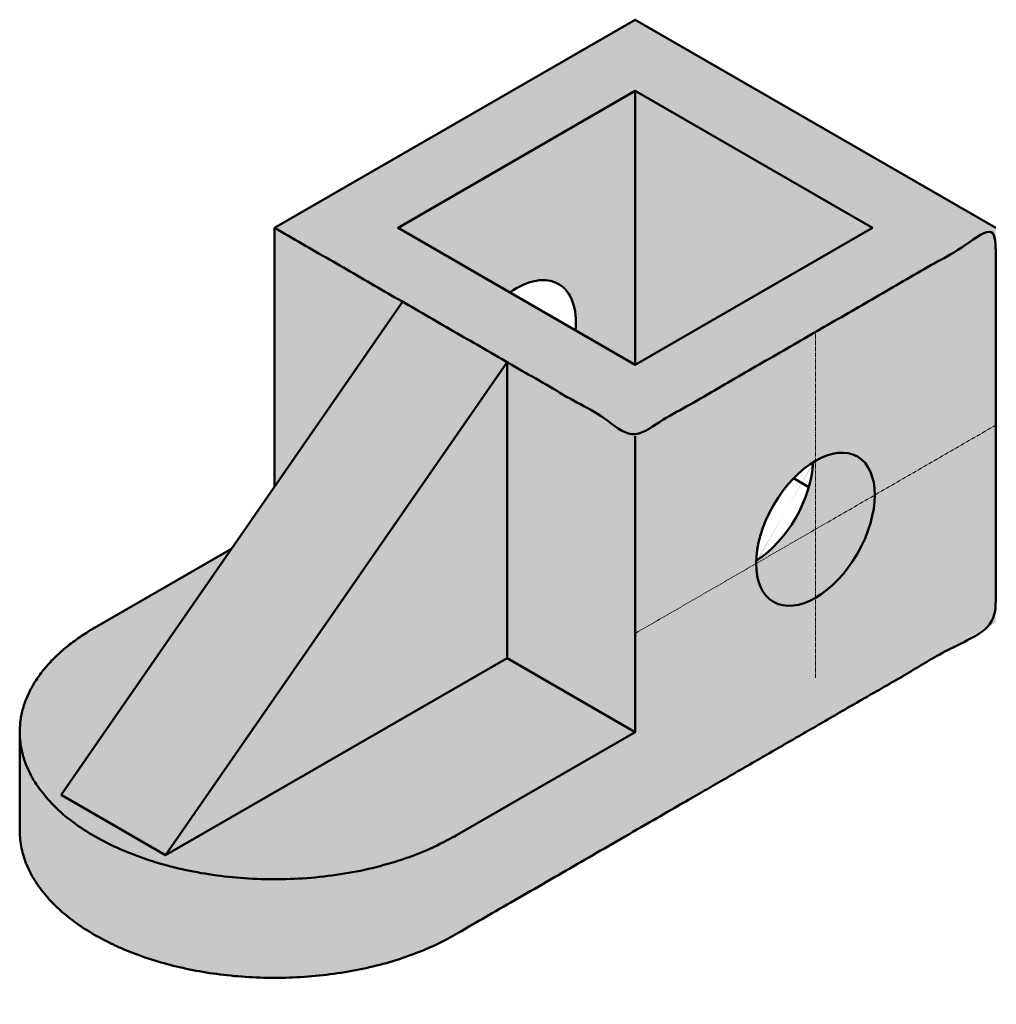
# Model space of a CAD drawing. Units: millimetres. Extents: x -10 to 168, y 10 to 190.
import ezdxf

# ---------------------------------------------------------------- set-up
doc = ezdxf.new("R2010")
doc.units = ezdxf.units.MM
doc.header["$MEASUREMENT"] = 0
doc.linetypes.add('CENTER2', pattern=[1.125, 0.75, -0.125, 0.125, -0.125])
for name, color, linetype, lineweight in [('M-CNTR', 4, 'CENTER2', 18), ('M-HATC', 7, 'Continuous', 18), ('M-OUTL', 7, 'Continuous', 50)]:
    doc.layers.add(name, color=color, linetype=linetype, lineweight=lineweight)

msp = doc.modelspace()

# ---------------------------------------------------------------- hatches: boundary and pattern name
at = {"layer": 'M-HATC'}
h = msp.add_hatch(color=256, dxfattribs=at)
h.set_gradient(color1=(229, 232, 120), color2=(229, 232, 120), tint=1)
edge = h.paths.add_edge_path()
edge.add_line((102.0273422709656, 189.9473373900985), (36.2094115833483, 151.9473373900985))
edge.add_spline(control_points=[(36.20941158334833, 151.9473373900985), (47.88458083858976, 145.2066752777504), (59.55975009383122, 138.4660131654023)], knot_values=[7.001422800068761, 7.001422800068761, 7.001422800068761, 7.356194490192344, 7.356194490192344, 7.356194490192344], weights=[1, 1, 1], degree=2, periodic=0)
edge.add_spline(control_points=[(59.55975009383122, 138.4660131654023), (64.33906351049411, 135.7066752777504), (69.11837692715702, 132.9473373900985)], knot_values=[6.856194490192344, 6.856194490192344, 6.856194490192344, 7.001422800068761, 7.001422800068761, 7.001422800068761], weights=[1, 1, 1], degree=2, periodic=0)
edge.add_spline(control_points=[(69.11837692715702, 132.9473373900985), (73.88151664797141, 130.1973373900985), (78.6446563687858, 127.4473373900985)], knot_values=[6.711457648087082, 6.711457648087082, 6.711457648087082, 6.856194490192344, 6.856194490192344, 6.856194490192344], weights=[1, 1, 1], degree=2, periodic=0)
edge.add_spline(control_points=[(78.6446563687858, 127.4473373900985), (90.33599931987573, 120.6973373900985), (102.0273422709657, 113.9473373900985)], knot_values=[6.356194490192344, 6.356194490192344, 6.356194490192344, 6.711457648087082, 6.711457648087082, 6.711457648087082], weights=[1, 1, 1], degree=2, periodic=0)
edge.add_spline(control_points=[(102.0273422709657, 113.9473373900985), (118.48182494287, 123.4473373900985), (134.9363076147743, 132.9473373900985)], knot_values=[5.856194490192345, 5.856194490192345, 5.856194490192345, 6.356194490192345, 6.356194490192345, 6.356194490192345], weights=[1, 1, 1], degree=2, periodic=0)
edge.add_spline(control_points=[(134.9363076147743, 132.9473373900985), (151.3907902866787, 142.4473373900985), (167.845272958583, 151.9473373900985)], knot_values=[5.356194490192345, 5.356194490192345, 5.356194490192345, 5.856194490192345, 5.856194490192345, 5.856194490192345], weights=[1, 1, 1], degree=2, periodic=0)
edge.add_line((167.845272958583, 151.9473373900985), (102.0273422709656, 189.9473373900985))
h.paths.add_polyline_path([(145.3286124601876, 151.9473373900985), (102.0273422709657, 126.9473373900985), (58.72607208174374, 151.9473373900985), (102.0273422709656, 176.9473373900985)], flags=16)
edge = h.paths.add_edge_path()
edge.add_spline(control_points=[(167.845272958583, 115.9473373900985), (167.845272958583, 133.9473373900985), (167.845272958583, 151.9473373900985)], knot_values=[4.856194490192345, 4.856194490192345, 4.856194490192345, 5.356194490192345, 5.356194490192345, 5.356194490192345], weights=[1, 1, 1], degree=2, periodic=0)
edge.add_spline(control_points=[(167.845272958583, 151.9473373900985), (151.3907902866787, 142.4473373900985), (134.9363076147743, 132.9473373900985)], knot_values=[5.356194490192345, 5.356194490192345, 5.356194490192345, 5.856194490192345, 5.856194490192345, 5.856194490192345], weights=[1, 1, 1], degree=2, periodic=0)
edge.add_line((134.9363076147743, 132.9473373900985), (134.9363076147743, 109.4473373900985))
edge.add_ellipse((134.9363076147743, 96.94733739009851), major_axis=(-7.654655446197424, -13.25825214724778), ratio=0.577350269189626, start_angle=149.9999999999999, end_angle=210, ccw=False)
edge.add_line((145.7616251620798, 103.1973373900985), (167.845272958583, 115.9473373900985))
edge = h.paths.add_edge_path()
edge.add_spline(control_points=[(134.9363076147743, 132.9473373900985), (118.48182494287, 123.4473373900985), (102.0273422709657, 113.9473373900985)], knot_values=[5.856194490192345, 5.856194490192345, 5.856194490192345, 6.356194490192345, 6.356194490192345, 6.356194490192345], weights=[1, 1, 1], degree=2, periodic=0)
edge.add_line((102.0273422709656, 113.9473373900985), (102.0273422709657, 77.94733739009851))
edge.add_line((102.0273422709657, 77.94733739009851), (124.1064732416631, 90.6947295995037))
edge.add_ellipse((134.9363076147743, 96.94733739009851), major_axis=(-7.654655446197424, -13.25825214724778), ratio=0.577350269189626, start_angle=327.93073727587256, end_angle=329.99999999999994, ccw=False)
edge.add_ellipse((134.9363076147743, 96.94733739009851), major_axis=(-7.654655446197424, -13.25825214724778), ratio=0.577350269189626, start_angle=212.0692627241274, end_angle=327.93073727587256, ccw=False)
edge.add_line((134.9363076147743, 109.5003097916459), (134.9363076147743, 132.9473373900985))
edge = h.paths.add_edge_path()
edge.add_ellipse((134.9363076147743, 96.94733739009851), major_axis=(-7.654655446197424, -13.25825214724778), ratio=0.577350269189626, start_angle=329.99999999999994, end_angle=389.99999999999994, ccw=False)
edge.add_line((124.1109900674688, 90.69733739009851), (102.0273422709657, 77.94733739009851))
edge.add_line((102.0273422709657, 77.94733739009851), (102.0273422709656, 59.94733739009851))
edge.add_line((102.0273422709656, 59.94733739009851), (69.11837692715771, 40.94733739009922))
edge.add_spline(control_points=[(69.11837692715702, 40.94733739009853), (50.11837692715701, 29.97768227549562), (24.16389425525267, 33.99285471819417), (-1.790588416651686, 38.00802716089272), (-8.745071088556024, 52.99285471819417), (-10.330893529532, 56.409827185539), (-10.33089352953207, 59.9473373900982)], knot_values=[1.78086055689268, 1.78086055689268, 1.78086055689268, 2.828058108089279, 2.828058108089279, 3.875255659285876, 3.875255659285876, 4.141592653589794, 4.141592653589794, 4.141592653589794], weights=[1, 0.8660254037844385, 1, 0.8660254037844385, 1, 0.9659258262890698, 0.9491840326991372], degree=2, periodic=0)
edge.add_spline(control_points=[(-10.33089352953207, 59.94733739009851), (-10.33089352953207, 50.94733739009851), (-10.33089352953207, 41.9473373900985)], knot_values=[0, 0, 0, 1, 1, 1], weights=[1, 1, 1], degree=2, periodic=0)
edge.add_spline(control_points=[(-10.33089352953207, 41.9473373900985), (-10.33089352953208, 23.99333884526288), (18.39920787943271, 17.12264105744734), (47.12930928839751, 10.25194326963181), (69.11837692715702, 22.94733739009852)], knot_values=[1, 1, 1, 2.178097245096171, 2.178097245096171, 3.356194490192345, 3.356194490192345, 3.356194490192345], weights=[1, 0.831469612302545, 1, 0.831469612302545, 1], degree=2, periodic=0)
edge.add_spline(control_points=[(69.11837692715702, 22.94733739009852), (118.48182494287, 51.44733739009851), (167.845272958583, 79.94733739009851)], knot_values=[3.356194490192345, 3.356194490192345, 3.356194490192345, 4.356194490192345, 4.356194490192345, 4.356194490192345], weights=[1, 1, 1], degree=2, periodic=0)
edge.add_spline(control_points=[(167.845272958583, 79.94733739009851), (167.845272958583, 97.94733739009851), (167.845272958583, 115.9473373900985)], knot_values=[4.356194490192345, 4.356194490192345, 4.356194490192345, 4.856194490192345, 4.856194490192345, 4.856194490192345], weights=[1, 1, 1], degree=2, periodic=0)
edge.add_line((167.845272958583, 115.9473373900985), (145.7616251620798, 103.1973373900985))
edge.add_ellipse((134.9363076147743, 96.94733739009851), major_axis=(-7.654655446197424, -13.25825214724778), ratio=0.577350269189626, start_angle=29.999999999999886, end_angle=149.9999999999999, ccw=False)
edge = h.paths.add_edge_path()
edge.add_line((102.0273422709657, 77.94733739009851), (102.0273422709656, 113.9473373900985))
edge.add_spline(control_points=[(102.0273422709657, 113.9473373900985), (90.33599931987573, 120.6973373900985), (78.6446563687858, 127.4473373900985)], knot_values=[6.356194490192345, 6.356194490192345, 6.356194490192345, 6.711457648087082, 6.711457648087082, 6.711457648087082], weights=[1, 1, 1], degree=2, periodic=0)
edge.add_line((78.6446563687858, 127.4473373900985), (78.6446563687858, 73.4473373900985))
edge.add_line((78.6446563687858, 73.4473373900985), (102.0273422709656, 59.94733739009851))
edge.add_line((102.0273422709656, 59.94733739009851), (102.0273422709657, 77.94733739009851))
edge = h.paths.add_edge_path(flags=17)
edge.add_line((78.6446563687858, 73.44733739009848), (16.29082729630624, 37.44733739009851))
edge.add_line((16.29082729630624, 37.44733739009851), (-2.794078978648371, 48.46601316540233))
edge.add_line((-2.794078978648371, 48.46601316540233), (28.33970570199551, 93.4037605810563))
edge.add_line((28.33970570199551, 93.4037605810563), (3.300446239539809, 78.94733739009858))
edge.add_spline(control_points=[(3.300446239539661, 78.94733739009851), (-10.33089352953229, 71.07727970500959), (-10.33089352953207, 59.9473373900982)], knot_values=[1, 1, 1, 1.78086055689268, 1.78086055689268, 1.78086055689268], weights=[1, 0.9000995774953688, 0.9491840326991372], degree=2, periodic=0)
edge.add_spline(control_points=[(-10.33089352953207, 59.9473373900982), (-10.330893529532, 56.409827185539), (-8.745071088556024, 52.99285471819417), (-1.790588416651686, 38.00802716089272), (24.16389425525267, 33.99285471819417), (50.11837692715701, 29.97768227549562), (69.11837692715702, 40.94733739009853)], knot_values=[1.78086055689268, 1.78086055689268, 1.78086055689268, 2.047197551196598, 2.047197551196598, 3.094395102393195, 3.094395102393195, 4.141592653589794, 4.141592653589794, 4.141592653589794], weights=[0.9491840326991372, 0.9659258262890698, 1, 0.8660254037844385, 1, 0.8660254037844385, 1], degree=2, periodic=0)
edge.add_line((69.1183769271493, 40.94733739009451), (102.0273422709656, 59.94733739009851))
edge.add_line((102.0273422709656, 59.94733739009851), (78.6446563687858, 73.44733739009848))
h.paths.add_polyline_path([(78.6446563687858, 73.4473373900985), (78.6446563687858, 127.4473373900985), (16.29082729630627, 37.44733739009851)], flags=17)
edge = h.paths.add_edge_path()
edge.add_spline(control_points=[(78.6446563687858, 127.4473373900985), (73.88151664797141, 130.1973373900985), (69.11837692715702, 132.9473373900985)], knot_values=[6.711457648087082, 6.711457648087082, 6.711457648087082, 6.856194490192345, 6.856194490192345, 6.856194490192345], weights=[1, 1, 1], degree=2, periodic=0)
edge.add_spline(control_points=[(69.11837692715702, 132.9473373900985), (64.33906351049411, 135.7066752777504), (59.55975009383122, 138.4660131654023)], knot_values=[6.856194490192345, 6.856194490192345, 6.856194490192345, 7.001422800068762, 7.001422800068762, 7.001422800068762], weights=[1, 1, 1], degree=2, periodic=0)
edge.add_line((59.55975009383124, 138.4660131654023), (-2.794078978648343, 48.46601316540231))
edge.add_line((-2.794078978648343, 48.46601316540231), (16.29082729630624, 37.44733739009848))
edge.add_line((16.29082729630624, 37.44733739009848), (78.6446563687858, 127.4473373900985))
edge = h.paths.add_edge_path()
edge.add_spline(control_points=[(59.55975009383121, 138.4660131654023), (47.88458083858976, 145.2066752777503), (36.20941158334833, 151.9473373900985)], knot_values=[7.001422800068762, 7.001422800068762, 7.001422800068762, 7.356194490192345, 7.356194490192345, 7.356194490192345], weights=[1, 1, 1], degree=2, periodic=0)
edge.add_line((36.20941158334833, 151.9473373900985), (36.2094115833483, 104.7627026036618))
edge.add_line((36.2094115833483, 104.7627026036618), (59.55975009383121, 138.4660131654023))
edge = h.paths.add_edge_path(flags=16)
edge.add_line((102.0273422709656, 176.9473373900985), (58.72607208174371, 151.9473373900985))
edge.add_line((58.72607208174371, 151.9473373900985), (79.14766449006567, 140.156925515873))
edge.add_ellipse((80.37670717635469, 128.4473373900985), major_axis=(-7.654655446197424, -13.25825214724778), ratio=0.577350269189626, start_angle=504.0081530082931, end_angle=575.9918469917066, ccw=False)
edge.add_line((91.13202930427256, 133.237749264324), (102.0273422709657, 126.9473373900985))
edge.add_line((102.0273422709657, 126.9473373900985), (102.0273422709656, 176.9473373900985))
h.paths.add_polyline_path([(102.0273422709656, 176.9473373900985), (102.0273422709657, 126.9473373900985), (145.3286124601876, 151.9473373900985)], flags=0)
edge = h.paths.add_edge_path(flags=17)
edge.add_ellipse((134.9363076147743, 96.94733739009851), major_axis=(-7.654655446197424, -13.25825214724778), ratio=0.577350269189626, start_angle=149.9999999999999, end_angle=209.9999999999999)
edge.add_line((134.9363076147743, 109.4473373900985), (134.9363076147743, 96.94733739009851))
edge.add_line((134.9363076147743, 96.94733739009851), (145.7616251620798, 103.1973373900985))
edge = h.paths.add_edge_path(flags=17)
edge.add_ellipse((134.9363076147743, 96.94733739009851), major_axis=(-7.654655446197424, -13.25825214724778), ratio=0.577350269189626, start_angle=29.99999999999994, end_angle=149.9999999999999)
edge.add_line((145.7616251620798, 103.1973373900985), (134.9363076147743, 96.94733739009851))
edge.add_line((134.9363076147743, 96.94733739009851), (134.9363076147743, 84.44733739009853))
edge = h.paths.add_edge_path(flags=17)
edge.add_line((134.9363076147743, 96.94733739009851), (124.1109900674688, 90.6973373900985))
edge.add_ellipse((134.9363076147743, 96.94733739009851), major_axis=(-7.654655446197424, -13.25825214724778), ratio=0.577350269189626, start_angle=329.9999999999999, end_angle=390)
edge.add_line((134.9363076147743, 84.44733739009851), (134.9363076147743, 96.94733739009851))
edge = h.paths.add_edge_path(flags=17)
edge.add_ellipse((134.9363076147743, 96.94733739009851), major_axis=(-7.654655446197424, -13.25825214724778), ratio=0.577350269189626, start_angle=209.9999999999999, end_angle=212.0692627241273)
edge.add_ellipse((123.6779773655766, 103.4473373900985), major_axis=(-7.654655446197424, -13.25825214724778), ratio=0.577350269189626, start_angle=32.06926272412511, end_angle=147.930737275875, ccw=False)
edge.add_ellipse((134.9363076147743, 96.94733739009851), major_axis=(-7.654655446197424, -13.25825214724778), ratio=0.577350269189626, start_angle=327.9307372758725, end_angle=329.9999999999999)
edge.add_line((124.1109900674688, 90.6973373900985), (134.9363076147743, 96.94733739009851))
edge.add_line((134.9363076147743, 96.94733739009851), (134.9363076147743, 109.4473373900985))

# ---------------------------------------------------------------- linework, layer by layer
at = {"layer": 'M-CNTR'}
for p, q in [((69.11837692715699, 133.0673373900985), (69.11837692715699, 132.9473373900984)), ((134.9363076147743, 69.8273373900985), (134.9363076147743, 133.0673373900985)), ((102.0273422709657, 77.94733739009851), (167.9491960070371, 116.0073373900985))]:
    msp.add_line(p, q, dxfattribs=at)
at = {"layer": 'M-OUTL'}
for p, q in [((59.55975009383122, 138.4660131654023), (-2.794078978648344, 48.46601316540232)), ((133.7376544026982, 104.638829229813), (130.9380687323864, 106.255170770187)), ((3.30044623953966, 78.94733739009851), (28.33970570199553, 93.4037605810563)), ((69.118376927157, 40.94733739009852), (102.0273422709656, 59.94733739009851)), ((-2.794078978648354, 48.46601316540233), (16.29082729630626, 37.44733739009851))]:
    msp.add_line(p, q, dxfattribs=at)
for points in [[(167.845272958583, 151.9473373900985), (102.0273422709656, 189.9473373900985), (36.20941158334832, 151.9473373900985), (36.20941158334832, 104.7627026036618)], [(102.0273422709657, 126.9473373900985), (58.72607208174372, 151.9473373900985), (102.0273422709656, 176.9473373900985), (102.0273422709657, 126.9473373900985), (145.3286124601876, 151.9473373900985), (102.0273422709656, 176.9473373900985)], [(78.6446563687858, 73.4473373900985), (102.0273422709656, 59.94733739009851), (102.0273422709656, 113.9473373900985)]]:
    msp.add_lwpolyline(points, dxfattribs=at)
msp.add_lwpolyline([(78.6446563687858, 127.4473373900985), (78.6446563687858, 73.44733739009848), (16.29082729630626, 37.44733739009851)], close=True, dxfattribs=at)
for centre, start_param, end_param in [((80.37670717635469, 128.4473373900985), 8.525600362565482, 10.32395555897327), ((123.6779773655766, 103.4473373900985), 0.8262435778150166, 2.315349075774776)]:
    msp.add_ellipse(centre, major_axis=(-7.654655446197419, -13.25825214724777), ratio=0.577350269189626, start_param=start_param, end_param=end_param, dxfattribs=at)
msp.add_ellipse((134.9363076147743, 96.94733739009851), major_axis=(-7.654655446197419, -13.25825214724777), ratio=0.577350269189626, dxfattribs=at)
for points, weights, knots in [([(-10.33089352953207, 59.94733739009851), (-10.33089352953207, 50.94733739009851), (-10.33089352953207, 41.9473373900985), (-10.33089352953208, 23.99333884526288), (18.39920787943271, 17.12264105744734), (47.12930928839751, 10.25194326963181), (69.11837692715702, 22.94733739009852), (118.48182494287, 51.44733739009851), (167.845272958583, 79.94733739009851), (167.845272958583, 115.9473373900985), (167.845272958583, 151.9473373900985), (134.9363076147743, 132.9473373900985), (102.0273422709657, 113.9473373900985), (69.118376927157, 132.9473373900984), (36.20941158334833, 151.9473373900985)], [1, 1, 1, 0.831469612302545, 1, 0.831469612302545, 1, 1, 1, 1, 1, 1, 1, 1, 1], [0, 0, 0, 1, 1, 2.178097245096171, 2.178097245096171, 3.356194490192345, 3.356194490192345, 4.356194490192345, 4.356194490192345, 5.356194490192345, 5.356194490192345, 6.356194490192345, 6.356194490192345, 7.356194490192345, 7.356194490192345, 7.356194490192345]), ([(3.19652319108551, 79.00733739009851), (3.248484715312586, 78.97733739009851), (3.300446239539661, 78.94733739009851), (-15.69955376046036, 67.97768227549562), (-8.745071088556024, 52.99285471819417), (-1.790588416651686, 38.00802716089272), (24.16389425525267, 33.99285471819417), (50.11837692715701, 29.97768227549562), (69.11837692715702, 40.94733739009853), (69.17033845138405, 40.91733739009851), (69.22229997561112, 40.88733739009851)], [1, 1, 1, 0.8660254037844385, 1, 0.8660254037844385, 1, 0.8660254037844385, 1, 1, 1], [0, 0, 0, 1, 1, 2.047197551196598, 2.047197551196598, 3.094395102393195, 3.094395102393195, 4.141592653589794, 4.141592653589794, 5.141592653589794, 5.141592653589794, 5.141592653589794])]:
    msp.add_rational_spline(points, weights, degree=2, knots=knots, dxfattribs=at)

doc.saveas('drawing.dxf')
